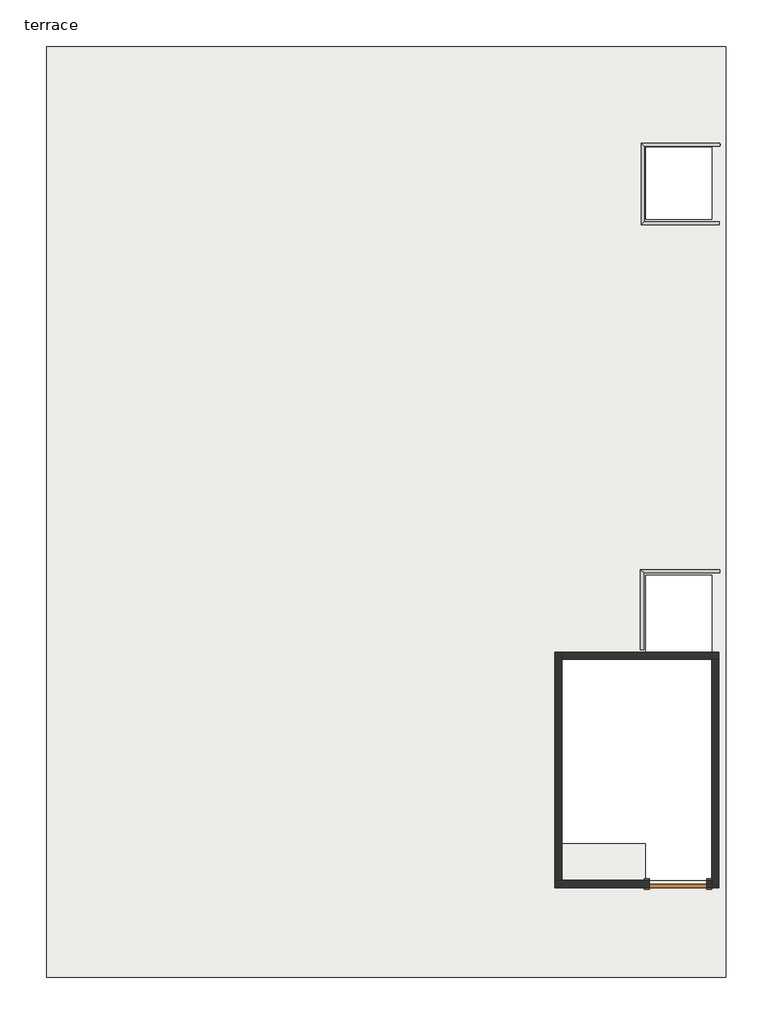
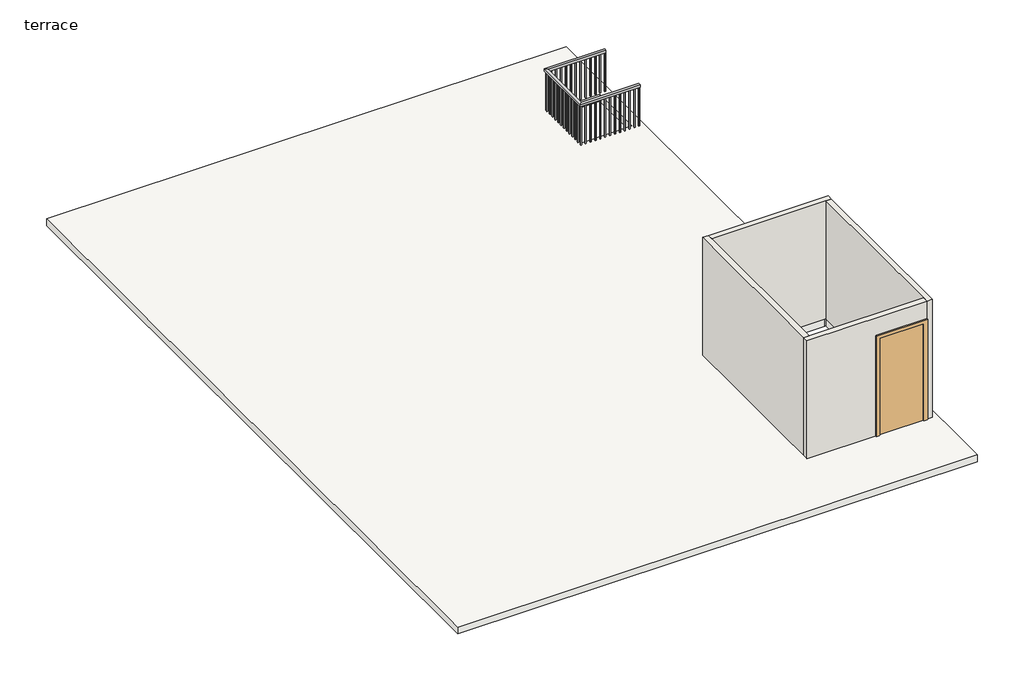
# One storey, incomplete: 4 walls, 2 railings, 1 door, 1 slab.
"""IFC4 building model written with IfcOpenShell, lengths in millimetres."""

from ifc_helpers import new_model, si_unit, frame, origin, place, context, project, spatial, polyline, outline, extrude, faceted_brep, transform, mapped, element, save
from components import door_e5f9f3c4

model = new_model("IFC4")

# Units and contexts
model_context = context("Model", 3, world=origin())
ifc_project = project(units=[si_unit("LENGTHUNIT", "METRE", prefix="MILLI")], contexts=[model_context])

# Site, building, storey
site = spatial("IfcSite", under=ifc_project)
building = spatial("IfcBuilding", under=site)
storey = spatial("IfcBuildingStorey", under=building, Name="terrace", Elevation=10210.8)

# Door
placement = place(None, origin())
door_shape = door_e5f9f3c4(model_context)
element("IfcDoor", 1, ObjectType="Single-Flush : 36\" x 84\"", at=placement, inside=storey, context=model_context, shape_type="MappedRepresentation", body=[
    mapped(door_shape, transform((1922.6501403, -490.0742075, 10210.8), x_axis=(-1.0, 0.0, 0.0), y_axis=(0.0, -1.0, 0.0), z_axis=(0.0, 0.0, 1.0))),
])

# Railings
element("IfcRailing", 2, ObjectType="Handrail - Rectangular", at=placement, inside=storey, context=model_context, shape_type="SolidModel", body=[
    faceted_brep([(2588.4250073, 11270.6841594, 11125.2), (2588.4250073, 11219.8841594, 11125.2), (2588.4250073, 11219.8841594, 11074.4), (2588.4250073, 11270.6841594, 11074.4), (1340.261267, 11270.6841594, 11074.4), (1340.261267, 11270.6841594, 11125.2), (1391.061267, 11219.8841594, 11074.4), (1391.061267, 11219.8841594, 11125.2), (2578.511267, 9975.2841594, 11125.2), (2578.511267, 9975.2841594, 11074.4), (2578.511267, 10026.0841594, 11074.4), (2578.511267, 10026.0841594, 11125.2), (1340.261267, 9975.2841594, 11125.2), (1340.261267, 9975.2841594, 11074.4), (1391.061267, 10026.0841594, 11074.4), (1391.061267, 10026.0841594, 11125.2)], [[[0, 1, 2, 3]], [[4, 5, 0, 3]], [[6, 4, 3, 2]], [[7, 6, 2, 1]], [[5, 7, 1, 0]], [[8, 9, 10, 11]], [[9, 8, 12, 13]], [[10, 9, 13, 14]], [[11, 10, 14, 15]], [[8, 11, 15, 12]], [[13, 12, 5, 4]], [[14, 13, 4, 6]], [[15, 14, 6, 7]], [[12, 15, 7, 5]]]),
    extrude(outline(polyline([(2575.336267, 11235.7591594), (2575.336267, 11254.8091594), (2594.386267, 11254.8091594), (2594.386267, 11235.7591594), (2575.336267, 11235.7591594)])), frame((0.0, 0.0, 10210.8), z_axis=(0.0, 0.0, 1.0), x_axis=(1.0, 0.0, 0.0)), (0.0, 0.0, 1.0), 863.6),
    extrude(outline(polyline([(2473.736267, 11235.7591594), (2473.736267, 11254.8091594), (2492.786267, 11254.8091594), (2492.786267, 11235.7591594), (2473.736267, 11235.7591594)])), frame((0.0, 0.0, 10210.8), z_axis=(0.0, 0.0, 1.0), x_axis=(1.0, 0.0, 0.0)), (0.0, 0.0, 1.0), 863.6),
    extrude(outline(polyline([(2372.136267, 11235.7591594), (2372.136267, 11254.8091594), (2391.186267, 11254.8091594), (2391.186267, 11235.7591594), (2372.136267, 11235.7591594)])), frame((0.0, 0.0, 10210.8), z_axis=(0.0, 0.0, 1.0), x_axis=(1.0, 0.0, 0.0)), (0.0, 0.0, 1.0), 863.6),
    extrude(outline(polyline([(2270.536267, 11235.7591594), (2270.536267, 11254.8091594), (2289.586267, 11254.8091594), (2289.586267, 11235.7591594), (2270.536267, 11235.7591594)])), frame((0.0, 0.0, 10210.8), z_axis=(0.0, 0.0, 1.0), x_axis=(1.0, 0.0, 0.0)), (0.0, 0.0, 1.0), 863.6),
    extrude(outline(polyline([(2168.936267, 11235.7591594), (2168.936267, 11254.8091594), (2187.986267, 11254.8091594), (2187.986267, 11235.7591594), (2168.936267, 11235.7591594)])), frame((0.0, 0.0, 10210.8), z_axis=(0.0, 0.0, 1.0), x_axis=(1.0, 0.0, 0.0)), (0.0, 0.0, 1.0), 863.6),
    extrude(outline(polyline([(2067.336267, 11235.7591594), (2067.336267, 11254.8091594), (2086.386267, 11254.8091594), (2086.386267, 11235.7591594), (2067.336267, 11235.7591594)])), frame((0.0, 0.0, 10210.8), z_axis=(0.0, 0.0, 1.0), x_axis=(1.0, 0.0, 0.0)), (0.0, 0.0, 1.0), 863.6),
    extrude(outline(polyline([(1965.736267, 11235.7591594), (1965.736267, 11254.8091594), (1984.786267, 11254.8091594), (1984.786267, 11235.7591594), (1965.736267, 11235.7591594)])), frame((0.0, 0.0, 10210.8), z_axis=(0.0, 0.0, 1.0), x_axis=(1.0, 0.0, 0.0)), (0.0, 0.0, 1.0), 863.6),
    extrude(outline(polyline([(1864.136267, 11235.7591594), (1864.136267, 11254.8091594), (1883.186267, 11254.8091594), (1883.186267, 11235.7591594), (1864.136267, 11235.7591594)])), frame((0.0, 0.0, 10210.8), z_axis=(0.0, 0.0, 1.0), x_axis=(1.0, 0.0, 0.0)), (0.0, 0.0, 1.0), 863.6),
    extrude(outline(polyline([(1762.536267, 11235.7591594), (1762.536267, 11254.8091594), (1781.586267, 11254.8091594), (1781.586267, 11235.7591594), (1762.536267, 11235.7591594)])), frame((0.0, 0.0, 10210.8), z_axis=(0.0, 0.0, 1.0), x_axis=(1.0, 0.0, 0.0)), (0.0, 0.0, 1.0), 863.6),
    extrude(outline(polyline([(1660.936267, 11235.7591594), (1660.936267, 11254.8091594), (1679.986267, 11254.8091594), (1679.986267, 11235.7591594), (1660.936267, 11235.7591594)])), frame((0.0, 0.0, 10210.8), z_axis=(0.0, 0.0, 1.0), x_axis=(1.0, 0.0, 0.0)), (0.0, 0.0, 1.0), 863.6),
    extrude(outline(polyline([(1559.336267, 11235.7591594), (1559.336267, 11254.8091594), (1578.386267, 11254.8091594), (1578.386267, 11235.7591594), (1559.336267, 11235.7591594)])), frame((0.0, 0.0, 10210.8), z_axis=(0.0, 0.0, 1.0), x_axis=(1.0, 0.0, 0.0)), (0.0, 0.0, 1.0), 863.6),
    extrude(outline(polyline([(1457.736267, 11235.7591594), (1457.736267, 11254.8091594), (1476.786267, 11254.8091594), (1476.786267, 11235.7591594), (1457.736267, 11235.7591594)])), frame((0.0, 0.0, 10210.8), z_axis=(0.0, 0.0, 1.0), x_axis=(1.0, 0.0, 0.0)), (0.0, 0.0, 1.0), 863.6),
    extrude(outline(polyline([(1375.186267, 11210.3591594), (1356.136267, 11210.3591594), (1356.136267, 11229.4091594), (1375.186267, 11229.4091594), (1375.186267, 11210.3591594)])), frame((0.0, 0.0, 10210.8), z_axis=(0.0, 0.0, 1.0), x_axis=(1.0, 0.0, 0.0)), (0.0, 0.0, 1.0), 863.6),
    extrude(outline(polyline([(1375.186267, 11108.7591594), (1356.136267, 11108.7591594), (1356.136267, 11127.8091594), (1375.186267, 11127.8091594), (1375.186267, 11108.7591594)])), frame((0.0, 0.0, 10210.8), z_axis=(0.0, 0.0, 1.0), x_axis=(1.0, 0.0, 0.0)), (0.0, 0.0, 1.0), 863.6),
    extrude(outline(polyline([(1375.186267, 11007.1591594), (1356.136267, 11007.1591594), (1356.136267, 11026.2091594), (1375.186267, 11026.2091594), (1375.186267, 11007.1591594)])), frame((0.0, 0.0, 10210.8), z_axis=(0.0, 0.0, 1.0), x_axis=(1.0, 0.0, 0.0)), (0.0, 0.0, 1.0), 863.6),
    extrude(outline(polyline([(1375.186267, 10905.5591594), (1356.136267, 10905.5591594), (1356.136267, 10924.6091594), (1375.186267, 10924.6091594), (1375.186267, 10905.5591594)])), frame((0.0, 0.0, 10210.8), z_axis=(0.0, 0.0, 1.0), x_axis=(1.0, 0.0, 0.0)), (0.0, 0.0, 1.0), 863.6),
    extrude(outline(polyline([(1375.186267, 10803.9591594), (1356.136267, 10803.9591594), (1356.136267, 10823.0091594), (1375.186267, 10823.0091594), (1375.186267, 10803.9591594)])), frame((0.0, 0.0, 10210.8), z_axis=(0.0, 0.0, 1.0), x_axis=(1.0, 0.0, 0.0)), (0.0, 0.0, 1.0), 863.6),
    extrude(outline(polyline([(1375.186267, 10702.3591594), (1356.136267, 10702.3591594), (1356.136267, 10721.4091594), (1375.186267, 10721.4091594), (1375.186267, 10702.3591594)])), frame((0.0, 0.0, 10210.8), z_axis=(0.0, 0.0, 1.0), x_axis=(1.0, 0.0, 0.0)), (0.0, 0.0, 1.0), 863.6),
    extrude(outline(polyline([(1375.186267, 10600.7591594), (1356.136267, 10600.7591594), (1356.136267, 10619.8091594), (1375.186267, 10619.8091594), (1375.186267, 10600.7591594)])), frame((0.0, 0.0, 10210.8), z_axis=(0.0, 0.0, 1.0), x_axis=(1.0, 0.0, 0.0)), (0.0, 0.0, 1.0), 863.6),
    extrude(outline(polyline([(1375.186267, 10499.1591594), (1356.136267, 10499.1591594), (1356.136267, 10518.2091594), (1375.186267, 10518.2091594), (1375.186267, 10499.1591594)])), frame((0.0, 0.0, 10210.8), z_axis=(0.0, 0.0, 1.0), x_axis=(1.0, 0.0, 0.0)), (0.0, 0.0, 1.0), 863.6),
    extrude(outline(polyline([(1375.186267, 10397.5591594), (1356.136267, 10397.5591594), (1356.136267, 10416.6091594), (1375.186267, 10416.6091594), (1375.186267, 10397.5591594)])), frame((0.0, 0.0, 10210.8), z_axis=(0.0, 0.0, 1.0), x_axis=(1.0, 0.0, 0.0)), (0.0, 0.0, 1.0), 863.6),
    extrude(outline(polyline([(1375.186267, 10295.9591594), (1356.136267, 10295.9591594), (1356.136267, 10315.0091594), (1375.186267, 10315.0091594), (1375.186267, 10295.9591594)])), frame((0.0, 0.0, 10210.8), z_axis=(0.0, 0.0, 1.0), x_axis=(1.0, 0.0, 0.0)), (0.0, 0.0, 1.0), 863.6),
    extrude(outline(polyline([(1375.186267, 10194.3591594), (1356.136267, 10194.3591594), (1356.136267, 10213.4091594), (1375.186267, 10213.4091594), (1375.186267, 10194.3591594)])), frame((0.0, 0.0, 10210.8), z_axis=(0.0, 0.0, 1.0), x_axis=(1.0, 0.0, 0.0)), (0.0, 0.0, 1.0), 863.6),
    extrude(outline(polyline([(1375.186267, 10092.7591594), (1356.136267, 10092.7591594), (1356.136267, 10111.8091594), (1375.186267, 10111.8091594), (1375.186267, 10092.7591594)])), frame((0.0, 0.0, 10210.8), z_axis=(0.0, 0.0, 1.0), x_axis=(1.0, 0.0, 0.0)), (0.0, 0.0, 1.0), 863.6),
    extrude(outline(polyline([(1470.436267, 10010.2091594), (1470.436267, 9991.1591594), (1451.386267, 9991.1591594), (1451.386267, 10010.2091594), (1470.436267, 10010.2091594)])), frame((0.0, 0.0, 10210.8), z_axis=(0.0, 0.0, 1.0), x_axis=(1.0, 0.0, 0.0)), (0.0, 0.0, 1.0), 863.6),
    extrude(outline(polyline([(1572.036267, 10010.2091594), (1572.036267, 9991.1591594), (1552.986267, 9991.1591594), (1552.986267, 10010.2091594), (1572.036267, 10010.2091594)])), frame((0.0, 0.0, 10210.8), z_axis=(0.0, 0.0, 1.0), x_axis=(1.0, 0.0, 0.0)), (0.0, 0.0, 1.0), 863.6),
    extrude(outline(polyline([(1673.636267, 10010.2091594), (1673.636267, 9991.1591594), (1654.586267, 9991.1591594), (1654.586267, 10010.2091594), (1673.636267, 10010.2091594)])), frame((0.0, 0.0, 10210.8), z_axis=(0.0, 0.0, 1.0), x_axis=(1.0, 0.0, 0.0)), (0.0, 0.0, 1.0), 863.6),
    extrude(outline(polyline([(1775.236267, 10010.2091594), (1775.236267, 9991.1591594), (1756.186267, 9991.1591594), (1756.186267, 10010.2091594), (1775.236267, 10010.2091594)])), frame((0.0, 0.0, 10210.8), z_axis=(0.0, 0.0, 1.0), x_axis=(1.0, 0.0, 0.0)), (0.0, 0.0, 1.0), 863.6),
    extrude(outline(polyline([(1876.836267, 10010.2091594), (1876.836267, 9991.1591594), (1857.786267, 9991.1591594), (1857.786267, 10010.2091594), (1876.836267, 10010.2091594)])), frame((0.0, 0.0, 10210.8), z_axis=(0.0, 0.0, 1.0), x_axis=(1.0, 0.0, 0.0)), (0.0, 0.0, 1.0), 863.6),
    extrude(outline(polyline([(1978.436267, 10010.2091594), (1978.436267, 9991.1591594), (1959.386267, 9991.1591594), (1959.386267, 10010.2091594), (1978.436267, 10010.2091594)])), frame((0.0, 0.0, 10210.8), z_axis=(0.0, 0.0, 1.0), x_axis=(1.0, 0.0, 0.0)), (0.0, 0.0, 1.0), 863.6),
    extrude(outline(polyline([(2080.036267, 10010.2091594), (2080.036267, 9991.1591594), (2060.986267, 9991.1591594), (2060.986267, 10010.2091594), (2080.036267, 10010.2091594)])), frame((0.0, 0.0, 10210.8), z_axis=(0.0, 0.0, 1.0), x_axis=(1.0, 0.0, 0.0)), (0.0, 0.0, 1.0), 863.6),
    extrude(outline(polyline([(2181.636267, 10010.2091594), (2181.636267, 9991.1591594), (2162.586267, 9991.1591594), (2162.586267, 10010.2091594), (2181.636267, 10010.2091594)])), frame((0.0, 0.0, 10210.8), z_axis=(0.0, 0.0, 1.0), x_axis=(1.0, 0.0, 0.0)), (0.0, 0.0, 1.0), 863.6),
    extrude(outline(polyline([(2283.236267, 10010.2091594), (2283.236267, 9991.1591594), (2264.186267, 9991.1591594), (2264.186267, 10010.2091594), (2283.236267, 10010.2091594)])), frame((0.0, 0.0, 10210.8), z_axis=(0.0, 0.0, 1.0), x_axis=(1.0, 0.0, 0.0)), (0.0, 0.0, 1.0), 863.6),
    extrude(outline(polyline([(2384.836267, 10010.2091594), (2384.836267, 9991.1591594), (2365.786267, 9991.1591594), (2365.786267, 10010.2091594), (2384.836267, 10010.2091594)])), frame((0.0, 0.0, 10210.8), z_axis=(0.0, 0.0, 1.0), x_axis=(1.0, 0.0, 0.0)), (0.0, 0.0, 1.0), 863.6),
    extrude(outline(polyline([(2486.436267, 10010.2091594), (2486.436267, 9991.1591594), (2467.386267, 9991.1591594), (2467.386267, 10010.2091594), (2486.436267, 10010.2091594)])), frame((0.0, 0.0, 10210.8), z_axis=(0.0, 0.0, 1.0), x_axis=(1.0, 0.0, 0.0)), (0.0, 0.0, 1.0), 863.6),
    extrude(outline(polyline([(1375.186267, 11235.7591594), (1356.136267, 11235.7591594), (1356.136267, 11254.8091594), (1375.186267, 11254.8091594), (1375.186267, 11235.7591594)])), frame((0.0, 0.0, 10210.8), z_axis=(0.0, 0.0, 1.0), x_axis=(1.0, 0.0, 0.0)), (0.0, 0.0, 1.0), 863.6),
    extrude(outline(polyline([(1375.186267, 10010.2091594), (1375.186267, 9991.1591594), (1356.136267, 9991.1591594), (1356.136267, 10010.2091594), (1375.186267, 10010.2091594)])), frame((0.0, 0.0, 10210.8), z_axis=(0.0, 0.0, 1.0), x_axis=(1.0, 0.0, 0.0)), (0.0, 0.0, 1.0), 863.6),
    extrude(outline(polyline([(2569.3750073, 11235.7591594), (2569.3750073, 11254.8091594), (2588.4250073, 11254.8091594), (2588.4250073, 11235.7591594), (2569.3750073, 11235.7591594)])), frame((0.0, 0.0, 10210.8), z_axis=(0.0, 0.0, 1.0), x_axis=(1.0, 0.0, 0.0)), (0.0, 0.0, 1.0), 863.6),
    extrude(outline(polyline([(2578.511267, 10010.2091594), (2578.511267, 9991.1591594), (2559.461267, 9991.1591594), (2559.461267, 10010.2091594), (2578.511267, 10010.2091594)])), frame((0.0, 0.0, 10210.8), z_axis=(0.0, 0.0, 1.0), x_axis=(1.0, 0.0, 0.0)), (0.0, 0.0, 1.0), 863.6),
])
element("IfcRailing", 3, ObjectType="Handrail - Rectangular", at=placement, inside=storey, context=model_context, shape_type="SolidModel", body=[
    faceted_brep([(1326.083415, 3232.0136165, 11125.2), (1326.083415, 3232.0136165, 11074.4), (1376.883415, 3232.0136165, 11074.4), (1376.883415, 3232.0136165, 11125.2), (1326.083415, 4502.0136165, 11125.2), (1326.083415, 4502.0136165, 11074.4), (1376.883415, 4451.2136165, 11074.4), (1376.883415, 4451.2136165, 11125.2), (2588.4250073, 4502.0136165, 11125.2), (2588.4250073, 4451.2136165, 11125.2), (2588.4250073, 4451.2136165, 11074.4), (2588.4250073, 4502.0136165, 11074.4)], [[[0, 1, 2, 3]], [[1, 0, 4, 5]], [[2, 1, 5, 6]], [[3, 2, 6, 7]], [[0, 3, 7, 4]], [[8, 9, 10, 11]], [[5, 4, 8, 11]], [[6, 5, 11, 10]], [[7, 6, 10, 9]], [[4, 7, 9, 8]]]),
    extrude(outline(polyline([(2561.158415, 4467.0886165), (2561.158415, 4486.1386165), (2580.208415, 4486.1386165), (2580.208415, 4467.0886165), (2561.158415, 4467.0886165)])), frame((0.0, 0.0, 10210.8), z_axis=(0.0, 0.0, 1.0), x_axis=(1.0, 0.0, 0.0)), (0.0, 0.0, 1.0), 863.6),
    extrude(outline(polyline([(2459.558415, 4467.0886165), (2459.558415, 4486.1386165), (2478.608415, 4486.1386165), (2478.608415, 4467.0886165), (2459.558415, 4467.0886165)])), frame((0.0, 0.0, 10210.8), z_axis=(0.0, 0.0, 1.0), x_axis=(1.0, 0.0, 0.0)), (0.0, 0.0, 1.0), 863.6),
    extrude(outline(polyline([(2357.958415, 4467.0886165), (2357.958415, 4486.1386165), (2377.008415, 4486.1386165), (2377.008415, 4467.0886165), (2357.958415, 4467.0886165)])), frame((0.0, 0.0, 10210.8), z_axis=(0.0, 0.0, 1.0), x_axis=(1.0, 0.0, 0.0)), (0.0, 0.0, 1.0), 863.6),
    extrude(outline(polyline([(2256.358415, 4467.0886165), (2256.358415, 4486.1386165), (2275.408415, 4486.1386165), (2275.408415, 4467.0886165), (2256.358415, 4467.0886165)])), frame((0.0, 0.0, 10210.8), z_axis=(0.0, 0.0, 1.0), x_axis=(1.0, 0.0, 0.0)), (0.0, 0.0, 1.0), 863.6),
    extrude(outline(polyline([(2154.758415, 4467.0886165), (2154.758415, 4486.1386165), (2173.808415, 4486.1386165), (2173.808415, 4467.0886165), (2154.758415, 4467.0886165)])), frame((0.0, 0.0, 10210.8), z_axis=(0.0, 0.0, 1.0), x_axis=(1.0, 0.0, 0.0)), (0.0, 0.0, 1.0), 863.6),
    extrude(outline(polyline([(2053.158415, 4467.0886165), (2053.158415, 4486.1386165), (2072.208415, 4486.1386165), (2072.208415, 4467.0886165), (2053.158415, 4467.0886165)])), frame((0.0, 0.0, 10210.8), z_axis=(0.0, 0.0, 1.0), x_axis=(1.0, 0.0, 0.0)), (0.0, 0.0, 1.0), 863.6),
    extrude(outline(polyline([(1951.558415, 4467.0886165), (1951.558415, 4486.1386165), (1970.608415, 4486.1386165), (1970.608415, 4467.0886165), (1951.558415, 4467.0886165)])), frame((0.0, 0.0, 10210.8), z_axis=(0.0, 0.0, 1.0), x_axis=(1.0, 0.0, 0.0)), (0.0, 0.0, 1.0), 863.6),
    extrude(outline(polyline([(1849.958415, 4467.0886165), (1849.958415, 4486.1386165), (1869.008415, 4486.1386165), (1869.008415, 4467.0886165), (1849.958415, 4467.0886165)])), frame((0.0, 0.0, 10210.8), z_axis=(0.0, 0.0, 1.0), x_axis=(1.0, 0.0, 0.0)), (0.0, 0.0, 1.0), 863.6),
    extrude(outline(polyline([(1748.358415, 4467.0886165), (1748.358415, 4486.1386165), (1767.408415, 4486.1386165), (1767.408415, 4467.0886165), (1748.358415, 4467.0886165)])), frame((0.0, 0.0, 10210.8), z_axis=(0.0, 0.0, 1.0), x_axis=(1.0, 0.0, 0.0)), (0.0, 0.0, 1.0), 863.6),
    extrude(outline(polyline([(1646.758415, 4467.0886165), (1646.758415, 4486.1386165), (1665.808415, 4486.1386165), (1665.808415, 4467.0886165), (1646.758415, 4467.0886165)])), frame((0.0, 0.0, 10210.8), z_axis=(0.0, 0.0, 1.0), x_axis=(1.0, 0.0, 0.0)), (0.0, 0.0, 1.0), 863.6),
    extrude(outline(polyline([(1545.158415, 4467.0886165), (1545.158415, 4486.1386165), (1564.208415, 4486.1386165), (1564.208415, 4467.0886165), (1545.158415, 4467.0886165)])), frame((0.0, 0.0, 10210.8), z_axis=(0.0, 0.0, 1.0), x_axis=(1.0, 0.0, 0.0)), (0.0, 0.0, 1.0), 863.6),
    extrude(outline(polyline([(1443.558415, 4467.0886165), (1443.558415, 4486.1386165), (1462.608415, 4486.1386165), (1462.608415, 4467.0886165), (1443.558415, 4467.0886165)])), frame((0.0, 0.0, 10210.8), z_axis=(0.0, 0.0, 1.0), x_axis=(1.0, 0.0, 0.0)), (0.0, 0.0, 1.0), 863.6),
    extrude(outline(polyline([(1361.008415, 4441.6886165), (1341.958415, 4441.6886165), (1341.958415, 4460.7386165), (1361.008415, 4460.7386165), (1361.008415, 4441.6886165)])), frame((0.0, 0.0, 10210.8), z_axis=(0.0, 0.0, 1.0), x_axis=(1.0, 0.0, 0.0)), (0.0, 0.0, 1.0), 863.6),
    extrude(outline(polyline([(1361.008415, 4340.0886165), (1341.958415, 4340.0886165), (1341.958415, 4359.1386165), (1361.008415, 4359.1386165), (1361.008415, 4340.0886165)])), frame((0.0, 0.0, 10210.8), z_axis=(0.0, 0.0, 1.0), x_axis=(1.0, 0.0, 0.0)), (0.0, 0.0, 1.0), 863.6),
    extrude(outline(polyline([(1361.008415, 4238.4886165), (1341.958415, 4238.4886165), (1341.958415, 4257.5386165), (1361.008415, 4257.5386165), (1361.008415, 4238.4886165)])), frame((0.0, 0.0, 10210.8), z_axis=(0.0, 0.0, 1.0), x_axis=(1.0, 0.0, 0.0)), (0.0, 0.0, 1.0), 863.6),
    extrude(outline(polyline([(1361.008415, 4136.8886165), (1341.958415, 4136.8886165), (1341.958415, 4155.9386165), (1361.008415, 4155.9386165), (1361.008415, 4136.8886165)])), frame((0.0, 0.0, 10210.8), z_axis=(0.0, 0.0, 1.0), x_axis=(1.0, 0.0, 0.0)), (0.0, 0.0, 1.0), 863.6),
    extrude(outline(polyline([(1361.008415, 4035.2886165), (1341.958415, 4035.2886165), (1341.958415, 4054.3386165), (1361.008415, 4054.3386165), (1361.008415, 4035.2886165)])), frame((0.0, 0.0, 10210.8), z_axis=(0.0, 0.0, 1.0), x_axis=(1.0, 0.0, 0.0)), (0.0, 0.0, 1.0), 863.6),
    extrude(outline(polyline([(1361.008415, 3933.6886165), (1341.958415, 3933.6886165), (1341.958415, 3952.7386165), (1361.008415, 3952.7386165), (1361.008415, 3933.6886165)])), frame((0.0, 0.0, 10210.8), z_axis=(0.0, 0.0, 1.0), x_axis=(1.0, 0.0, 0.0)), (0.0, 0.0, 1.0), 863.6),
    extrude(outline(polyline([(1361.008415, 3832.0886165), (1341.958415, 3832.0886165), (1341.958415, 3851.1386165), (1361.008415, 3851.1386165), (1361.008415, 3832.0886165)])), frame((0.0, 0.0, 10210.8), z_axis=(0.0, 0.0, 1.0), x_axis=(1.0, 0.0, 0.0)), (0.0, 0.0, 1.0), 863.6),
    extrude(outline(polyline([(1361.008415, 3730.4886165), (1341.958415, 3730.4886165), (1341.958415, 3749.5386165), (1361.008415, 3749.5386165), (1361.008415, 3730.4886165)])), frame((0.0, 0.0, 10210.8), z_axis=(0.0, 0.0, 1.0), x_axis=(1.0, 0.0, 0.0)), (0.0, 0.0, 1.0), 863.6),
    extrude(outline(polyline([(1361.008415, 3628.8886165), (1341.958415, 3628.8886165), (1341.958415, 3647.9386165), (1361.008415, 3647.9386165), (1361.008415, 3628.8886165)])), frame((0.0, 0.0, 10210.8), z_axis=(0.0, 0.0, 1.0), x_axis=(1.0, 0.0, 0.0)), (0.0, 0.0, 1.0), 863.6),
    extrude(outline(polyline([(1361.008415, 3527.2886165), (1341.958415, 3527.2886165), (1341.958415, 3546.3386165), (1361.008415, 3546.3386165), (1361.008415, 3527.2886165)])), frame((0.0, 0.0, 10210.8), z_axis=(0.0, 0.0, 1.0), x_axis=(1.0, 0.0, 0.0)), (0.0, 0.0, 1.0), 863.6),
    extrude(outline(polyline([(1361.008415, 3425.6886165), (1341.958415, 3425.6886165), (1341.958415, 3444.7386165), (1361.008415, 3444.7386165), (1361.008415, 3425.6886165)])), frame((0.0, 0.0, 10210.8), z_axis=(0.0, 0.0, 1.0), x_axis=(1.0, 0.0, 0.0)), (0.0, 0.0, 1.0), 863.6),
    extrude(outline(polyline([(1361.008415, 3324.0886165), (1341.958415, 3324.0886165), (1341.958415, 3343.1386165), (1361.008415, 3343.1386165), (1361.008415, 3324.0886165)])), frame((0.0, 0.0, 10210.8), z_axis=(0.0, 0.0, 1.0), x_axis=(1.0, 0.0, 0.0)), (0.0, 0.0, 1.0), 863.6),
    extrude(outline(polyline([(1361.008415, 4467.0886165), (1341.958415, 4467.0886165), (1341.958415, 4486.1386165), (1361.008415, 4486.1386165), (1361.008415, 4467.0886165)])), frame((0.0, 0.0, 10210.8), z_axis=(0.0, 0.0, 1.0), x_axis=(1.0, 0.0, 0.0)), (0.0, 0.0, 1.0), 863.6),
    extrude(outline(polyline([(2569.3750073, 4467.0886165), (2569.3750073, 4486.1386165), (2588.4250073, 4486.1386165), (2588.4250073, 4467.0886165), (2569.3750073, 4467.0886165)])), frame((0.0, 0.0, 10210.8), z_axis=(0.0, 0.0, 1.0), x_axis=(1.0, 0.0, 0.0)), (0.0, 0.0, 1.0), 863.6),
    extrude(outline(polyline([(1361.008415, 3232.0136165), (1341.958415, 3232.0136165), (1341.958415, 3251.0636165), (1361.008415, 3251.0636165), (1361.008415, 3232.0136165)])), frame((0.0, 0.0, 10210.8), z_axis=(0.0, 0.0, 1.0), x_axis=(1.0, 0.0, 0.0)), (0.0, 0.0, 1.0), 863.6),
])

# Slab
element("IfcSlab", 4, at=placement, inside=storey, context=model_context, shape_type="SweptSolid", body=[
    extrude(outline(polyline([(2684.6501403, 12806.8257925), (2684.6501403, -1973.1232395), (-8110.3498597, -1973.1232395), (-8110.3498597, 12806.8257925), (2684.6501403, 12806.8257925)]), holes=[polyline([(81.1501403, 3078.6257925), (81.1501403, 157.6257925), (1414.6501403, 157.6257925), (1414.6501403, -432.9242075), (2456.0501403, -432.9242075), (2456.0501403, 3078.6257925), (2430.6501403, 3078.6257925), (81.1501403, 3078.6257925)]), polyline([(2456.0501403, 10063.6257925), (2456.0501403, 11206.6257925), (1414.6501403, 11206.6257925), (1414.6501403, 10063.6257925), (2456.0501403, 10063.6257925)]), polyline([(2456.0501403, 3192.9257925), (2456.0501403, 4412.1257925), (1414.6501403, 4412.1257925), (1414.6501403, 3192.9257925), (2456.0501403, 3192.9257925)])]), frame((0.0, 0.0, 10058.4), z_axis=(0.0, 0.0, 1.0), x_axis=(1.0, 0.0, 0.0)), (0.0, 0.0, 1.0), 152.4),
])

# Walls
element("IfcWall", 5, at=placement, inside=storey, context=model_context, shape_type="Brep", body=[
    faceted_brep([(81.1501403, -432.9242075, 10210.8), (81.1501403, 3078.6257925, 10210.8), (81.1501403, 3192.9257925, 10210.8), (81.1501403, 3192.9257925, 12801.6), (81.1501403, 3078.6257925, 12801.6), (81.1501403, -432.9242075, 12801.6), (-33.1498597, -432.9242075, 10210.8), (-33.1498597, -432.9242075, 12801.6), (-33.1498597, 3192.9257925, 12801.6), (-33.1498597, 3192.9257925, 10210.8)], [[[0, 1, 2, 3, 4, 5]], [[6, 7, 8, 9]], [[2, 1, 0, 6, 9]], [[3, 2, 9, 8]], [[0, 5, 7, 6]], [[5, 4, 3, 8, 7]]]),
])
element("IfcWall", 6, at=placement, inside=storey, context=model_context, shape_type="Brep", body=[
    faceted_brep([(81.1501403, 3078.6257925, 10210.8), (2456.0501403, 3078.6257925, 10210.8), (2570.3501403, 3078.6257925, 10210.8), (2570.3501403, 3078.6257925, 12801.6), (2456.0501403, 3078.6257925, 12801.6), (81.1501403, 3078.6257925, 12801.6), (81.1501403, 3192.9257925, 10210.8), (81.1501403, 3192.9257925, 12801.6), (2570.3501403, 3192.9257925, 12801.6), (2570.3501403, 3192.9257925, 10210.8)], [[[0, 1, 2, 3, 4, 5]], [[6, 7, 8, 9]], [[2, 1, 0, 6, 9]], [[0, 5, 7, 6]], [[3, 2, 9, 8]], [[5, 4, 3, 8, 7]]]),
])
element("IfcWall", 7, at=placement, inside=storey, context=model_context, shape_type="Brep", body=[
    faceted_brep([(2456.0501403, 3078.6257925, 10210.8), (2456.0501403, -432.9242075, 10210.8), (2456.0501403, -547.2242075, 10210.8), (2456.0501403, -547.2242075, 12801.6), (2456.0501403, -432.9242075, 12801.6), (2456.0501403, 3078.6257925, 12801.6), (2570.3501403, 3078.6257925, 10210.8), (2570.3501403, 3078.6257925, 12801.6), (2570.3501403, -547.2242075, 12801.6), (2570.3501403, -547.2242075, 10210.8)], [[[0, 1, 2, 3, 4, 5]], [[6, 7, 8, 9]], [[2, 1, 0, 6, 9]], [[0, 5, 7, 6]], [[3, 2, 9, 8]], [[5, 4, 3, 8, 7]]]),
])
element("IfcWall", 8, at=placement, inside=storey, context=model_context, shape_type="Brep", body=[
    faceted_brep([(2456.0501403, -432.9242075, 12801.6), (2456.0501403, -432.9242075, 10210.8), (2379.8501403, -432.9242075, 10210.8), (2379.8501403, -432.9242075, 12344.4), (1465.4501403, -432.9242075, 12344.4), (1465.4501403, -432.9242075, 10210.8), (81.1501403, -432.9242075, 10210.8), (-33.1498597, -432.9242075, 10210.8), (-33.1498597, -432.9242075, 12801.6), (81.1501403, -432.9242075, 12801.6), (2456.0501403, -547.2242075, 10210.8), (2456.0501403, -547.2242075, 12801.6), (-33.1498597, -547.2242075, 12801.6), (-33.1498597, -547.2242075, 10210.8), (1465.4501403, -547.2242075, 10210.8), (1465.4501403, -547.2242075, 12344.4), (2379.8501403, -547.2242075, 12344.4), (2379.8501403, -547.2242075, 10210.8)], [[[0, 1, 2, 3, 4, 5, 6, 7, 8, 9]], [[10, 11, 12, 13, 14, 15, 16, 17]], [[1, 10, 17, 2]], [[13, 7, 6, 5, 14]], [[1, 0, 11, 10]], [[8, 7, 13, 12]], [[4, 15, 14, 5]], [[16, 3, 2, 17]], [[3, 16, 15, 4]], [[0, 9, 8, 12, 11]]]),
])

save(model, "model.ifc")

# Revit data of these elements
# Type "Single-Flush : 36\" x 84\""
#   Type Mark = "1"
#   Construction Type Id = "MDOOR"
#   Assembly Code = "C1020"
#   Analytic Construction = "Metal"
#   Thickness = 0' - 2"
#   Heat Transfer Coefficient (U) = 0.651978 BTU/(h·ft²·°F)
#   Height = 7' - 0"
#   Trim Projection Ext = 0' - 1"
#   Trim Projection Int = 0' - 1"
#   Trim Width = 0' - 3"
#   Width = 3' - 0"
#   Define Thermal Properties by = 1
#   Define Thermal Properties by = 1
#   Door Material = Door - Panel
#   Frame Material = Door - Frame
#   Visual Light Transmittance = 0
#   Solar Heat Gain Coefficient = 0
#   Function = (empty or 0)
#   Wall Closure = (empty or 0)
# Type "Handrail - Rectangular"
#   Assembly Code = "C2010400"
#   built-in parameter 1008612 = 0.0416667 (stored number, unit not read)
#   built-in parameter 1008611 = 0.0416667 (stored number, unit not read)
#   built-in parameter 1008609 = 0.333333 (stored number, unit not read)
#   built-in parameter 1008604 = 0.166667 (stored number, unit not read)
#   built-in parameter 1008603 = 0.166667 (stored number, unit not read)
#   Railing Height = 3' - 0"
#   built-in parameter 1008630 = 2
#   built-in parameter 1008610 = 2
#   built-in parameter 1008618 = Baluster - Square : 3/4"
# Type
#   Assembly Code = "B1010"
#   Function = 0
#   Layers, outside or top first: 0' - 6" "Concrete, Cast-in-Place gray" (function 1)
# Type
#   Assembly Code = "B2010"
#   Layers, outside or top first: 0' - 4 1/2" no material (function 1)
# Element 1 (IfcDoor, "Single-Flush : 36\" x 84\"")
#   Phase Created = New Construction
#   Materials on its faces: "Door - Frame", "Door - Panel"
# Elements 2, 3 (IfcRailing, "Handrail - Rectangular")
#   Phase Created = New Construction
# Element 4 (IfcSlab)
#   Height Offset From Level = 0' - 0"
#   Phase Created = New Construction
#   Materials on its faces: "Concrete, Cast-in-Place gray"
# Elements 5, 6, 7, 8 (IfcWall)
#   Top Offset = 0' - 0"
#   Base Offset = 0' - 0"
#   wall height = 8' - 6"
#   Phase Created = New Construction
#   Base Constraint = terrace
#   Materials on its faces: "Default Wall"
# Materials
#   "Door - Panel": class "Wood", colour RGB 210 159 95, transparency 0, Cost = 0
#   "Door - Frame": colour RGB 118 70 51, transparency 0, Cost = 0
#   "Concrete, Cast-in-Place gray": class "Concrete", colour RGB 192 192 192, transparency 0, Description = "Cast-in-place concrete", Cost = 0
#   "Default Wall": colour RGB 128 128 128, transparency 0, Cost = 0
